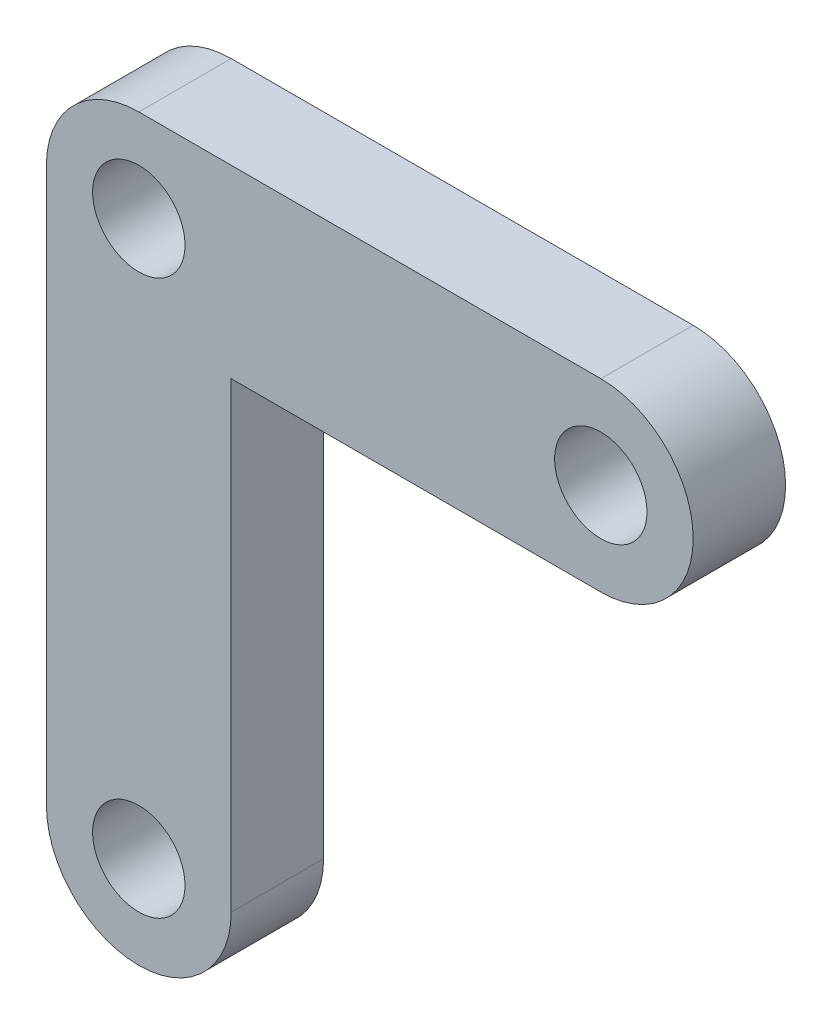
SolidWorks part; units mm, degrees
material "Plain Carbon Steel"
ref_plane "Front Plane" through (0, 0, 0) normal (0, 0, 1) x (1, 0, 0)
ref_plane "Top Plane" through (0, 0, 0) normal (0, 1, 0) x (1, 0, 0)
ref_plane "Right Plane" through (0, 0, 0) normal (1, 0, 0) x (0, 0, -1)
sketch "L-Link Profile" plane through (0, 0, 0) normal (0, 0, 1) x (1, 0, 0)
  line L0 (0, -30) -> (0, 0) construction
  line L1 (-5, -30) -> (-5, 0)
  line L2 (5, -30) -> (5, 0)
  line L3 (0, 0) -> (25, 0) construction
  line L4 (0, 5) -> (25, 5)
  line L5 (0, -5) -> (25, -5)
  arc A0 (-5, -30) -> (5, -30) centre (0, -30) ccw
  arc A1 (5, 0) -> (-5, 0) centre (0, 0) ccw
  arc A2 (0, 5) -> (0, -5) centre (0, 0) ccw
  arc A3 (25, -5) -> (25, 5) centre (25, 0) ccw
  circle A4 centre (0, 0) radius 2.5
  circle A5 centre (0, -30) radius 2.5
  circle A6 centre (25, 0) radius 2.5
  point P3 (0, -15)
  point P8 (12.5, 0)
  dimension "D3" = 5
  dimension "5" = 5
  dimension "D4" = 5
  dimension "D1" = 30
  dimension "D2" = 25
extrude "L-Link Plate 5mm" add sketch "L-Link Profile" along normal blind 5 contours L5 A3 L4 A1 L2 A6 | A2 L1 A0 L2 L5 A5 | A1 A2 L5 L2 A4
